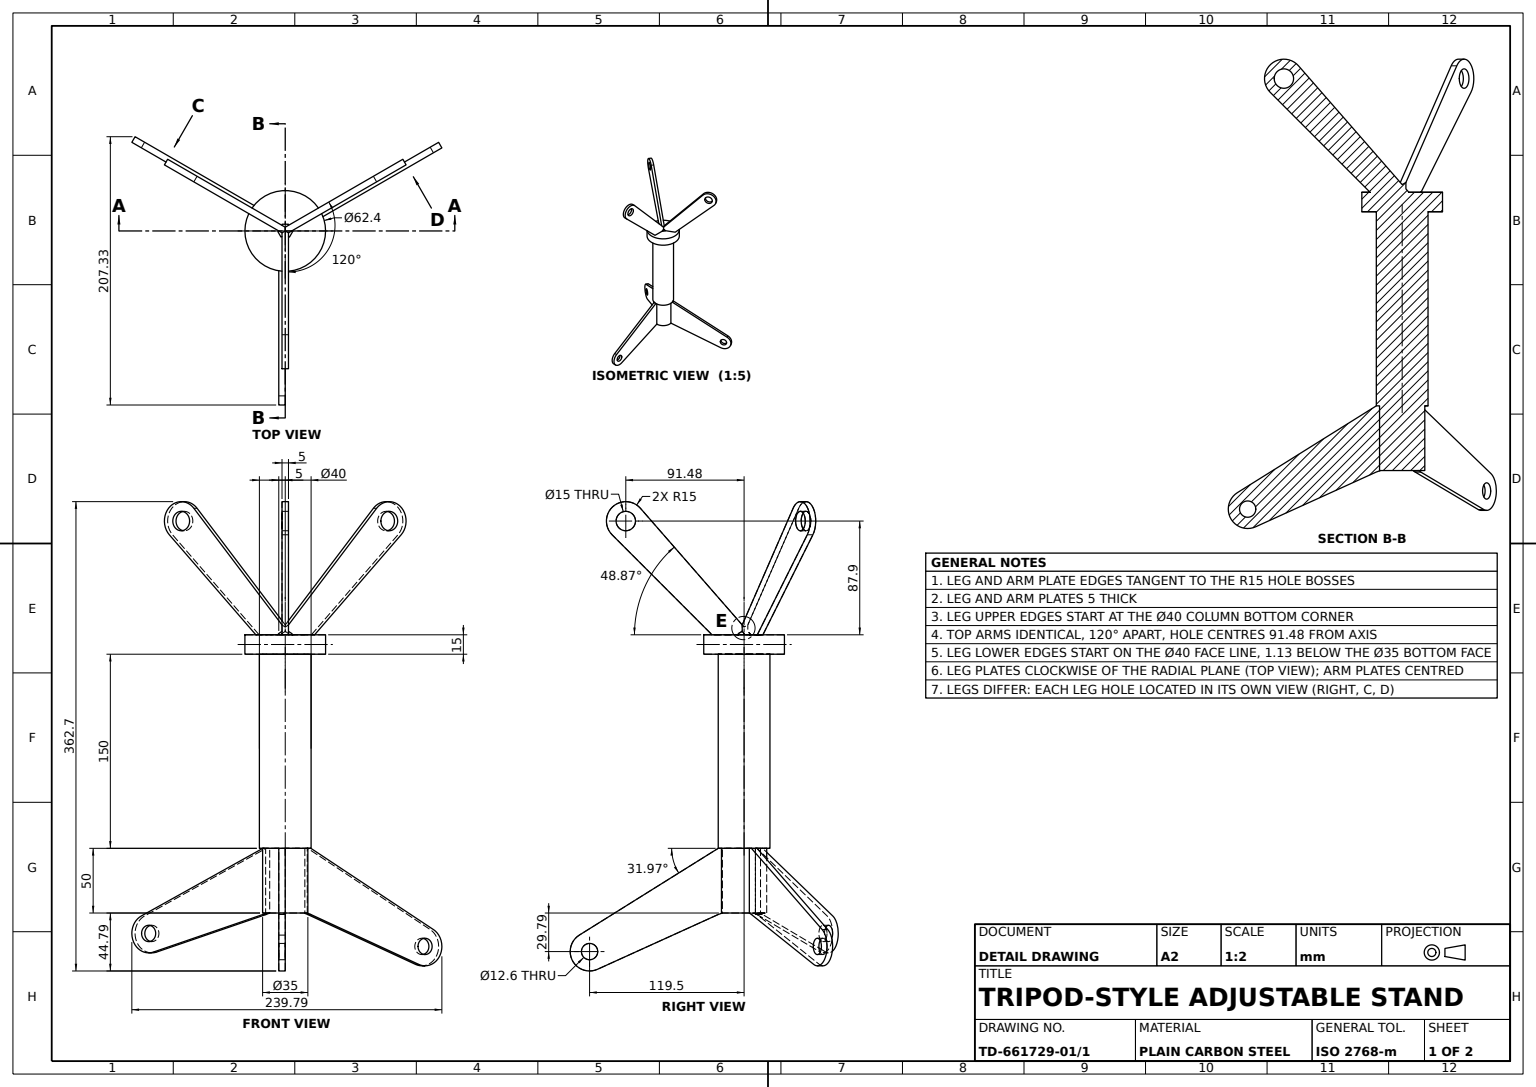
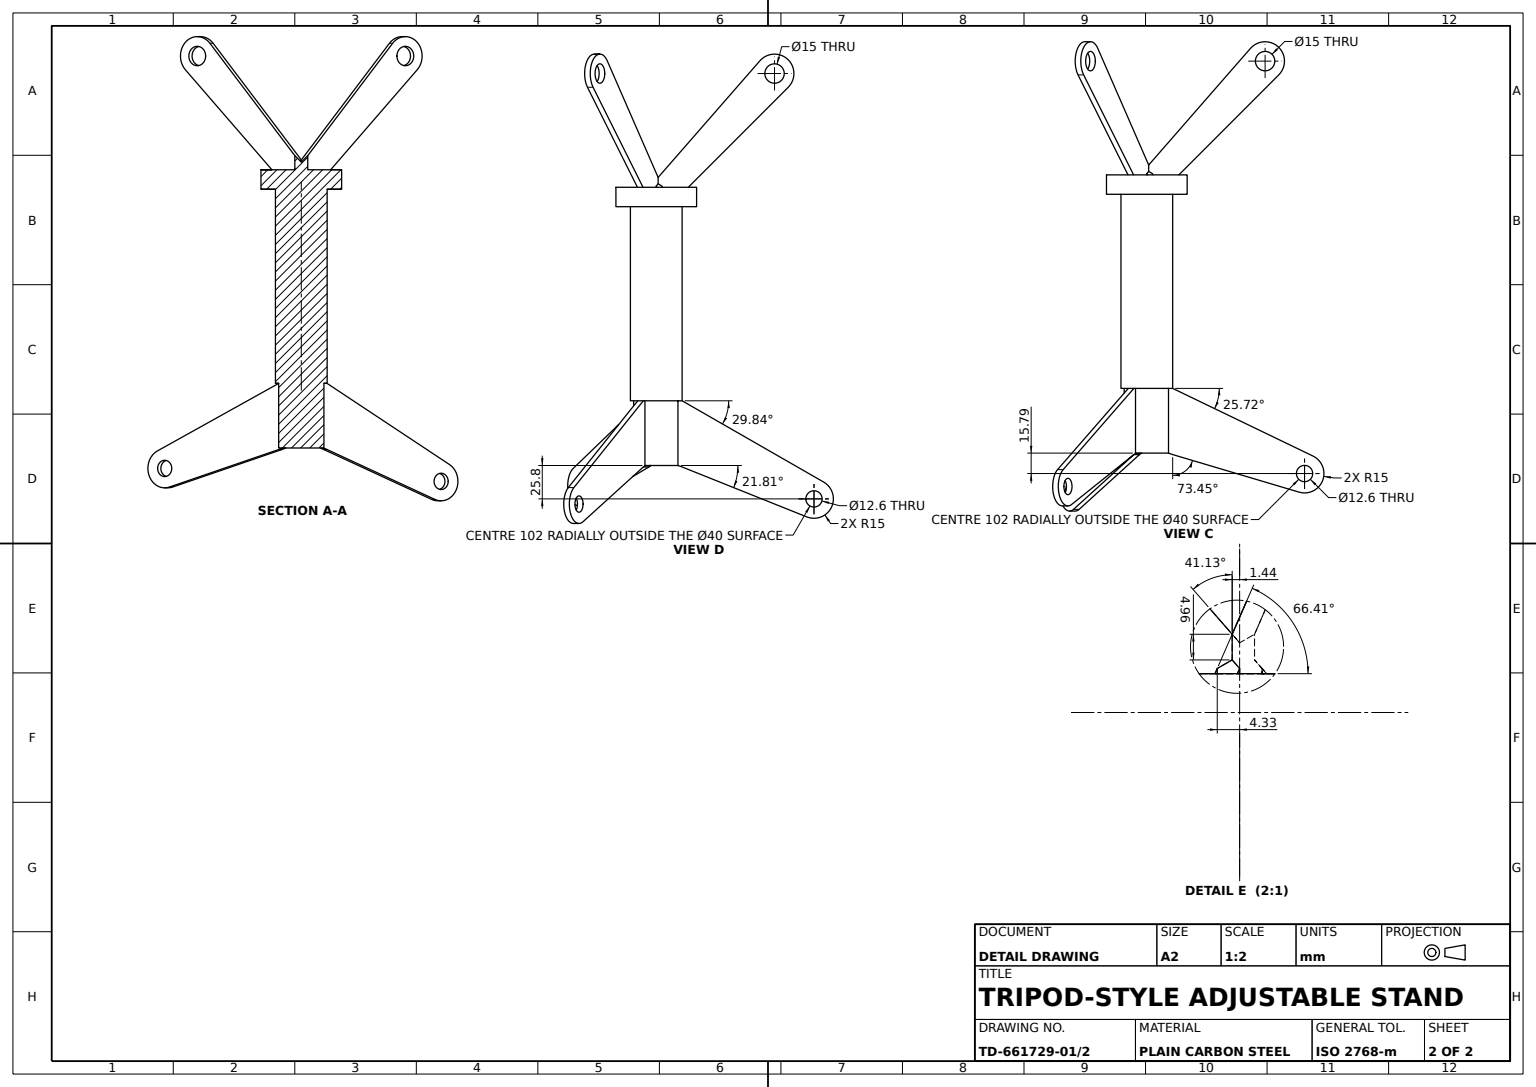
SolidWorks part; units mm, degrees
material "Plain Carbon Steel"
ref_plane "Front Plane" through (0, 0, 0) normal (0, 0, 1) x (1, 0, 0)
ref_plane "Top Plane" through (0, 0, 0) normal (0, 1, 0) x (1, 0, 0)
ref_plane "Right Plane" through (0, 0, 0) normal (1, 0, 0) x (0, 0, -1)
sketch "Column Sketch" plane through (0, 0, 0) normal (0, 1, 0) x (1, 0, 0)
  circle A0 centre (0, 0) radius 20
  dimension "D1" = 40
extrude "Column Ø40" add sketch "Column Sketch" along normal blind 150
sketch "Column Extension Sketch" plane through (0, 0, 0) normal (0, -1, 0) x (1, 0, 0)
  circle A0 centre (0, 0) radius 17.5
  dimension "D1" = 35
extrude "Column Extension Ø35" add sketch "Column Extension Sketch" along normal blind 50
sketch "Leg Plate Sketch" plane through (0, 0, 0) normal (0, 0, 1) x (1, 0, 0)
  line L0 (20, 0) -> (127.443, -67.0701)
  line L1 (113.3039, -93.4549) -> (20, -51.134)
  line L5 (-166.2173, -50) -> (131.2173, -50) construction
  line L6 (20, 0) -> (20, -51.134)
  arc A0 (127.443, -67.0701) -> (113.3039, -93.4549) centre (119.5, -79.7945) cw
  circle A1 centre (119.5, -79.7945) radius 6.3
  point P14 (-17.5, -50)
  point P15 (0, 0)
  dimension "D2" = 15
  dimension "D3" = 12.6
  dimension "D1" = 93.3039
  dimension "D4" = 99.5
  dimension "D5" = 107.443
extrude "Leg Plate" add sketch "Leg Plate Sketch" along normal blind 5 separate body
sketch "Leg Web Sketch" plane through (20, 0, 0) normal (-1, 0, 0) x (0, 0, 1)
  line L0 (5, 0) -> (0, 0) construction
  line L1 (5, 0) -> (5, -51.134) construction
  line L2 (0, 0) -> (0, -51.134) construction
  line L3 (5, -51.134) -> (0, -51.134) construction
  line L4 (5, 0) -> (0, 0)
  line L5 (5, 0) -> (5, -51.134)
  line L6 (0, 0) -> (0, -51.134)
  line L7 (5, -51.134) -> (0, -51.134)
extrude "Leg Web" add sketch "Leg Web Sketch" along normal up to surface (3.2295 mm away)
sketch "Leg Cut Sketch" plane through (0, 0, 5) normal (0, 0, 1) x (1, 0, 0)
  line L0 (20, -51.134) -> (16.7705, -50)
  line L1 (16.7705, -50) -> (16.7705, -51.134)
  line L2 (16.7705, -51.134) -> (20, -51.134)
extrude "Leg Cut" cut sketch "Leg Cut Sketch" against normal blind 22
pattern_circular "Leg Web Pattern 3x" count 3 over 360 about axis through (0, 0, 0) along (0, 1, 0) of "Leg Web"
pattern_circular "Leg Cut Pattern 3x" count 3 over 360 about axis through (0, 0, 0) along (0, 1, 0) of "Leg Cut"
sketch "Leg Boss A Sketch" plane through (4.3301, 0, -2.5) normal (0.866, 0, -0.5) x (-0.5, 0, -0.866)
  line L0 (20, -51.134) -> (116.4263, -89.7272)
  line L1 (129.4635, -62.7898) -> (20, 0)
  line L2 (20, 0) -> (20, 150) construction
  line L3 (20, 0) -> (20, -51.134)
  line L4 (20, -51.134) -> (20, 0) construction
  arc A0 (116.4263, -89.7272) -> (129.4635, -62.7898) centre (122, -75.8012) ccw
  circle A1 centre (122, -75.8012) radius 6.3
  dimension "D1" = 15
  dimension "D3" = 12.6
  dimension "D2" = 102
  dimension "D4" = 96.4263
extrude "Leg Boss A" add sketch "Leg Boss A Sketch" against normal up to surface (5 mm away) up to face at (-9.25, -30.278, -16.0215)
sketch "Leg Boss B Sketch" plane through (-4.3301, 0, -2.5) normal (-0.866, 0, -0.5) x (-0.5, 0, 0.866)
  line L0 (20, -51.134) -> (117.7284, -80.1666)
  line L1 (128.5101, -52.2741) -> (20, 0)
  line L2 (20, 0) -> (20, -51.134)
  line L3 (20, -51.134) -> (20, 0) construction
  arc A0 (117.7284, -80.1666) -> (128.5101, -52.2741) centre (122, -65.7877) ccw
  circle A1 centre (122, -65.7877) radius 6.3
  dimension "D1" = 15
  dimension "D3" = 12.6
  dimension "D2" = 102
  dimension "D4" = 97.7284
extrude "Leg Boss B" add sketch "Leg Boss B Sketch" against normal up to surface (5 mm away) up to face at (-9.25, -30.278, 16.0215)
sketch "Collar Sketch" plane through (0, 150, 0) normal (0, 1, 0) x (1, 0, 0)
  circle A0 centre (0, 0) radius 31.2
  dimension "D1" = 62.4
extrude "Collar Ø62.4" add sketch "Collar Sketch" along normal blind 15
sketch "Top Arm Sketch" plane through (0, 0, 0) normal (0, 0, 1) x (1, 0, 0)
  line L0 (-5.2078, 165) -> (80.1839, 262.7698)
  line L1 (31.2, 165) -> (-31.2, 165) construction
  line L2 (102.0882, 242.2959) -> (24.7922, 165)
  line L3 (24.7922, 165) -> (-5.2078, 165)
  arc A0 (80.1839, 262.7698) -> (102.0882, 242.2959) centre (91.4816, 252.9025) cw
  circle A1 centre (91.4816, 252.9025) radius 7.5
  point P9 (9.7922, 165)
  dimension "D3" = 15
  dimension "D5" = 15
  dimension "D1" = 30
  dimension "D2" = 120
  dimension "D4" = 45
  dimension "D6" = 9.7922
extrude "Top Arm" add sketch "Top Arm Sketch" along normal mid plane 5
pattern_circular "Top Arm Pattern 3x" count 3 over 360 about axis through (0, 0, 0) along (0, 1, 0) of "Top Arm"
